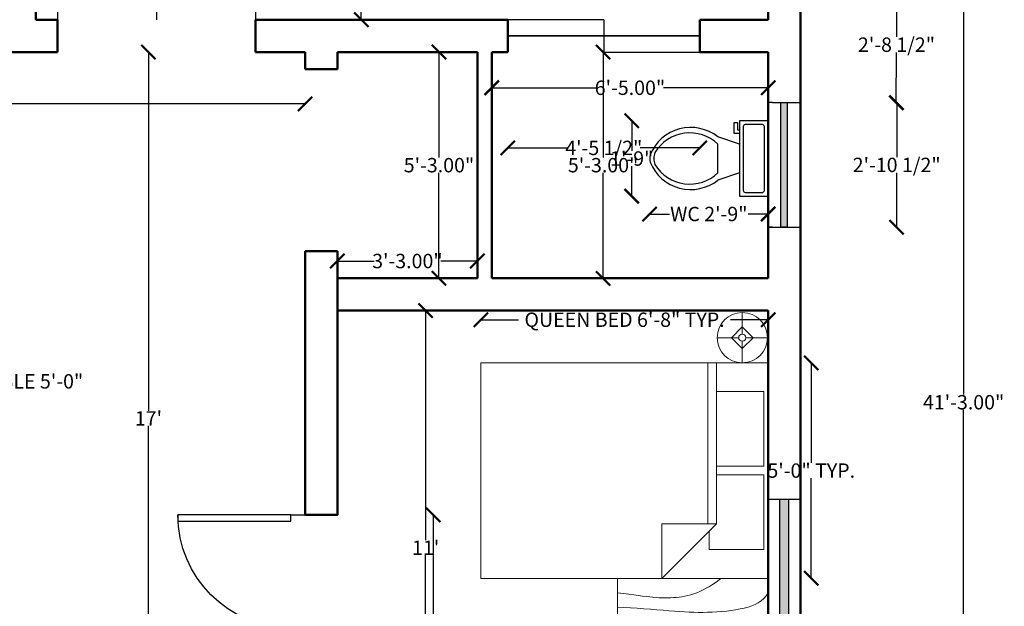
# Model space of a CAD drawing. Units: inches. Extents: x 2466 to 2986, y -30 to 527.
# Tile 4 of 5: x 2711 to 2986, y 190 to 354. Entities that reach past the tile are written whole.
import ezdxf

# ---------------------------------------------------------------- set-up
doc = ezdxf.new("R2010")
doc.units = ezdxf.units.IN
for name, color, linetype, lineweight in [('A-ANNO-DIMS', 2, 'Continuous', 18), ('A-FLOR-FIXT', 8, 'Continuous', 25), ('A-GLAZ', 4, 'Continuous', 25), ('A-GLAZ-PATT', 4, 'Continuous', 13), ('doors', 3, 'Continuous', 25), ('furniture', 6, 'Continuous', 18), ('walls', 40, 'Continuous', 50)]:
    doc.layers.add(name, color=color, linetype=linetype, lineweight=lineweight)
doc.styles.get("Standard").update_dxf_attribs({"font": 'arial.ttf'})
doc.dimstyles.get("Standard").update_dxf_attribs({"dimtxt": 4, "dimasz": 4, "dimexe": 0.18, "dimexo": 0.0625, "dimgap": 0.09, "dimtad": 0, "dimtih": 1, "dimtoh": 1, "dimzin": 0, "dimdsep": 46, "dimlunit": 3, "dimtxsty": 'Standard', "dimblk": 'ARCHTICK', "dimcen": 0.09, "dimse1": 1, "dimse2": 1, "dimclrd": 3, "dimclrt": 2, "dimadec": 0, "dimazin": 0, "dimtfac": 1, "dimtofl": 0, "dimtmove": 0, "dimatfit": 3, "dimfxl": 1, "dimtolj": 1, "dimtzin": 0, "dimarcsym": 0})

# ---------------------------------------------------------------- blocks, each defined once
blk = doc.blocks.new('*U8')
for p, q in [((0, 0), (0, -100)), ((700, 0), (700, -100))]:
    blk.add_line(p, q)
blk.add_lwpolyline([(0, 0), (0, 700), (43.75, 700), (43.75, 0)], close=True)
blk.add_arc((0, 0), 700, 0, 90)
blk = doc.blocks.new('Toilet - top')
for p, q in [((9.5, -6), (9.5, -2)), ((-8, -8.5), (-8, -8)), ((-7, -8), (-7, -9.5)), ((-4, -8), (-6, -14)), ((4, -8), (6, -14)), ((-10, -8.5), (-8, -8.5)), ((-10, -9.5), (-10, -8.5)), ((-7, -9.5), (-10, -9.5)), ((4, -14), (-4, -14))]:
    blk.add_line(p, q)
blk.add_lwpolyline([(10.5, -8), (10.5, 0), (-10.5, 0), (-10.5, -8)], close=True)
for points in [[(-9.5, -2), (-9.5, -6)], [(8.5, -1), (-8.5, -1)], [(-8.5, -7), (8.5, -7)]]:
    blk.add_lwpolyline(points)
for centre, radius, start, end in [((-8.62, -1.88), 0.884, 81.8699, 188.1301), ((8.62, -1.88), 0.884, 351.8699, 98.1301), ((-8.62, -6.12), 0.884, 171.8699, 278.1301), ((8.62, -6.12), 0.884, 261.8699, 8.1301), ((3.52, -21.58), 12.17, 141.4691, 247.9714), ((4.2, -21.82), 11.33, 136.3677, 238.9468), ((-3.52, -21.58), 12.17, 292.0284, 38.5307), ((-4.2, -21.82), 11.33, 301.053, 43.6321), ((0, -27.88), 4, 245.7318, 294.2682), ((0, -29), 4, 254.8605, 285.1395)]:
    blk.add_arc(centre, radius, start, end)
blk = doc.blocks.new('Bed - Queen')
for p, q in [((0, -80.00003), (0, 0)), ((0, 0), (59.99999, 0)), ((59.99999, 0), (59.99999, -80.00003)), ((7.99999, -1.2), (28.79998, -1.2)), ((7.99999, -14.4), (7.99999, -1.2)), ((28.79998, -1.2), (28.79998, -14.4)), ((31.19999, -1.2), (51.99999, -1.2)), ((31.19999, -14.4), (31.19999, -1.2)), ((51.99999, -1.2), (51.99999, -16.4)), ((0, -14.4), (44.8, -14.4)), ((59.99999, -29.6), (44.8, -14.4)), ((44.8, -14.4), (44.8, -29.6)), ((51.99999, -16.4), (46.79936, -16.4)), ((44.8, -16.8), (0, -16.8)), ((44.8, -29.6), (59.99999, -29.6)), ((59.99999, -80.00003), (0, -80.00003))]:
    blk.add_line(p, q)
blk = doc.blocks.new('Lamp - Table')
for p, q in [((0, 7), (0, 1)), ((0, 3), (-3, 0)), ((3, 0), (0, 3)), ((-1, 0), (-7, 0)), ((-3, 0), (0, -3)), ((0, -3), (3, 0)), ((1, 0), (7, 0)), ((0, -1), (0, -7))]:
    blk.add_line(p, q)
for radius in [7, 1]:
    blk.add_circle((0, 0), radius)
blk = doc.blocks.new('Table - Square Woodgrain 42 x 42 in.')
blk.add_line((0, -42), (42, -42))
for points in [[(0, -4), (1.704, -4.2172), (3.2358, -4.4188), (4.615, -4.604), (5.8615, -4.7721), (6.9951, -4.9224), (8.0357, -5.0541), (9.0031, -5.1667), (9.9171, -5.2594), (10.7951, -5.3316), (11.6445, -5.3836), (12.4702, -5.4157), (13.277, -5.4283), (14.0698, -5.4217), (14.8535, -5.3964), (15.6331, -5.3526), (16.4133, -5.2908), (17.1986, -5.2103), (17.9913, -5.1062), (18.793, -4.9727), (19.6056, -4.8038), (20.4307, -4.5937), (21.2701, -4.3365), (22.1256, -4.0262), (22.9989, -3.6571), (23.888, -3.2272), (24.7756, -2.7516), (25.6408, -2.2491), (26.4624, -1.7387), (27.2195, -1.2395), (27.891, -0.7703), (28.456, -0.3501), (28.8934, 0.002)], [(0, -42), (0, 0), (42, 0), (42, -42)], [(0, -8), (1.8203, -8.1001), (3.6741, -8.2149), (5.5411, -8.3408), (7.4011, -8.4741), (9.2339, -8.6112), (11.0193, -8.7484), (12.7371, -8.8821), (14.3671, -9.0086), (15.8954, -9.1246), (17.3337, -9.2278), (18.6997, -9.3159), (20.0116, -9.387), (21.2871, -9.4389), (22.5442, -9.4696), (23.8008, -9.477), (25.0749, -9.459), (26.3791, -9.4137), (27.7049, -9.3403), (29.0383, -9.2382), (30.3655, -9.1068), (31.6728, -8.9455), (32.9461, -8.7535), (34.1717, -8.5304), (35.3358, -8.2756), (36.4268, -7.9863), (37.443, -7.6521), (38.3849, -7.2603), (39.253, -6.7986), (40.048, -6.2542), (40.7705, -5.6147), (41.421, -4.8674), (42, -4)], [(42, -12), (39.1784, -12.8621), (36.4519, -13.5654), (33.8246, -14.1294), (31.3004, -14.5731), (28.8832, -14.9161), (26.577, -15.1775), (24.3858, -15.3768), (22.3136, -15.5332), (20.3622, -15.6632), (18.5254, -15.7718), (16.7947, -15.8612), (15.1618, -15.9338), (13.6183, -15.9916), (12.1558, -16.0369), (10.7659, -16.0718), (9.4403, -16.0987), (8.1703, -16.1191), (6.9461, -16.1325), (5.7577, -16.1377), (4.595, -16.1335), (3.4479, -16.1188), (2.3064, -16.0924), (1.1604, -16.0532), (0, -16)], [(42, -16), (37.6529, -16.7365), (33.8802, -17.329), (30.6179, -17.7961), (27.8015, -18.1561), (25.3668, -18.4275), (23.2497, -18.6288), (21.3859, -18.7785), (19.7111, -18.8949), (18.1693, -18.9939), (16.7375, -19.0795), (15.401, -19.1534), (14.1449, -19.217), (12.9544, -19.2717), (11.8148, -19.3191), (10.7113, -19.3606), (9.6291, -19.3976), (8.5534, -19.4323), (7.47, -19.4689), (6.3643, -19.5122), (5.222, -19.5672), (4.0288, -19.6386), (2.7703, -19.7313), (1.4321, -19.8501), (0, -20)], [(0, -24), (3.9243, -23.6805), (7.4766, -23.4138), (10.6891, -23.1954), (13.5943, -23.0205), (16.2247, -22.8847), (18.6125, -22.7832), (20.7903, -22.7116), (22.7903, -22.6651), (24.6563, -22.642), (26.4764, -22.6507), (28.35, -22.7024), (30.3766, -22.8084), (32.6555, -22.98), (35.2861, -23.2283), (38.3678, -23.5645), (42, -24)], [(42, -32), (37.392, -31.017), (33.4585, -30.2231), (30.1291, -29.5949), (27.3334, -29.109), (25.0009, -28.742), (23.0612, -28.4707), (21.4439, -28.2716), (20.0786, -28.1215), (18.8998, -28.0002), (17.8609, -27.9014), (16.9206, -27.8219), (16.0371, -27.7588), (15.1691, -27.709), (14.2748, -27.6693), (13.3128, -27.6368), (12.2415, -27.6083), (11.0295, -27.5824), (9.6867, -27.5643), (8.233, -27.5608), (6.6884, -27.5787), (5.0728, -27.6248), (3.4062, -27.7058), (1.7086, -27.8286), (0, -28)], [(0, -32), (5.4026, -32.5358), (9.9494, -33.019), (13.7424, -33.4553), (16.8834, -33.8505), (19.4743, -34.2106), (21.6171, -34.5413), (23.4136, -34.8486), (24.9657, -35.1382), (26.3614, -35.4156), (27.6332, -35.6841), (28.7995, -35.9467), (29.8788, -36.2064), (30.8897, -36.4661), (31.8507, -36.7288), (32.7802, -36.9973), (33.6968, -37.2747), (34.6175, -37.5635), (35.5531, -37.8651), (36.5128, -38.1805), (37.506, -38.5108), (38.5421, -38.8568), (39.6302, -39.2197), (40.7797, -39.6004), (42, -40)], [(0, -36), (3.0098, -36.2857), (5.5354, -36.5643), (7.6368, -36.8359), (9.374, -37.1009), (10.807, -37.3597), (11.9957, -37.6126), (13.0002, -37.8599), (13.8804, -38.102), (14.6874, -38.3393), (15.4365, -38.5729), (16.1338, -38.8041), (16.7858, -39.0341), (17.3987, -39.264), (17.9787, -39.4952), (18.5322, -39.7288), (19.0655, -39.9662), (19.5832, -40.2081), (20.0842, -40.4544), (20.5657, -40.7046), (21.0249, -40.9581), (21.459, -41.2144), (21.8653, -41.4731), (22.2409, -41.7335), (22.5831, -41.9951)]]:
    blk.add_lwpolyline(points)
blk = doc.blocks.new('*U18')
for p, q in [((0, 0), (0, -100)), ((800, 0), (800, -100))]:
    blk.add_line(p, q)
blk.add_lwpolyline([(0, 0), (0, 800), (43.75, 800), (43.75, 0)], close=True)
blk.add_arc((0, 0), 800, 0, 90)
blk = doc.blocks.new('_ArchTick')
at = {"color": 0, "linetype": 'ByBlock', "const_width": 0.15}
blk.add_lwpolyline([(-0.5, -0.5), (0.5, 0.5)], dxfattribs=at)
blk = doc.blocks.new('*D22')
at = {"layer": 'A-ANNO-DIMS', "color": 0, "lineweight": -2, "transparency": 16777216}
for p, q in [((2974.18, 494.8), (2974.18, 249.43)), ((2974.18, -0.2), (2974.18, 245.16))]:
    blk.add_line(p, q, dxfattribs=at)
at = {"layer": 'Defpoints', "color": 0, "transparency": 16777216}
for p in [(2928.73, 494.8), (2928.73, -0.2), (2974.18, -0.2)]:
    blk.add_point(p, dxfattribs=at)
at = {"layer": 'A-ANNO-DIMS', "color": 0, "lineweight": -2, "transparency": 16777216, "xscale": 4, "yscale": 4, "zscale": 4}
for p, rotation in [((2974.18, 494.8), 90), ((2974.18, -0.2), 270)]:
    blk.add_blockref('_ArchTick', p, dxfattribs=dict(at, rotation=rotation))
at = {"layer": 'A-ANNO-DIMS', "color": 0, "transparency": 16777216, "insert": (2974.18, 247.3), "char_height": 4, "attachment_point": 5}
blk.add_mtext('\\A1;41\'-3.00"', dxfattribs=at)
blk = doc.blocks.new('*D26')
at = {"layer": 'A-ANNO-DIMS', "color": 0, "lineweight": -2, "transparency": 16777216}
for p, q in [((2806.39, 485.8), (2806.39, 421.89)), ((2806.39, 353.8), (2806.39, 417.7))]:
    blk.add_line(p, q, dxfattribs=at)
at = {"layer": 'Defpoints', "color": 0, "transparency": 16777216}
for p in [(2715.73, 485.8), (2715.73, 353.8), (2806.39, 353.8)]:
    blk.add_point(p, dxfattribs=at)
at = {"layer": 'A-ANNO-DIMS', "color": 0, "lineweight": -2, "transparency": 16777216, "xscale": 4, "yscale": 4, "zscale": 4}
for p, rotation in [((2806.39, 485.8), 90), ((2806.39, 353.8), 270)]:
    blk.add_blockref('_ArchTick', p, dxfattribs=dict(at, rotation=rotation))
at = {"layer": 'A-ANNO-DIMS', "color": 0, "transparency": 16777216, "insert": (2806.39, 419.8), "char_height": 4, "attachment_point": 5}
blk.add_mtext("\\A1;11'", dxfattribs=at)
blk = doc.blocks.new('*D27')
at = {"layer": 'A-ANNO-DIMS', "color": 0, "lineweight": -2, "transparency": 16777216}
for p, q in [((2824.31, 272.8), (2824.31, 208.89)), ((2824.31, 140.8), (2824.31, 204.7))]:
    blk.add_line(p, q, dxfattribs=at)
at = {"layer": 'Defpoints', "color": 0, "transparency": 16777216}
for p in [(2799.73, 272.8), (2824.31, 272.8), (2799.73, 140.8)]:
    blk.add_point(p, dxfattribs=at)
at = {"layer": 'A-ANNO-DIMS', "color": 0, "lineweight": -2, "transparency": 16777216, "xscale": 4, "yscale": 4, "zscale": 4}
for p, rotation in [((2824.31, 272.8), 90), ((2824.31, 140.8), 270)]:
    blk.add_blockref('_ArchTick', p, dxfattribs=dict(at, rotation=rotation))
at = {"layer": 'A-ANNO-DIMS', "color": 0, "transparency": 16777216, "insert": (2824.31, 206.8), "char_height": 4, "attachment_point": 5}
blk.add_mtext("\\A1;11'", dxfattribs=at)
blk = doc.blocks.new('*D29')
at = {"layer": 'A-ANNO-DIMS', "color": 0, "lineweight": -2, "transparency": 16777216}
for p, q in [((2873.75, 344.8), (2873.75, 315.43)), ((2873.75, 281.8), (2873.75, 311.16))]:
    blk.add_line(p, q, dxfattribs=at)
at = {"layer": 'Defpoints', "color": 0, "transparency": 16777216}
for p in [(2842.73, 344.8), (2873.75, 344.8), (2842.73, 281.8)]:
    blk.add_point(p, dxfattribs=at)
at = {"layer": 'A-ANNO-DIMS', "color": 0, "lineweight": -2, "transparency": 16777216, "xscale": 4, "yscale": 4, "zscale": 4}
for p, rotation in [((2873.75, 344.8), 90), ((2873.75, 281.8), 270)]:
    blk.add_blockref('_ArchTick', p, dxfattribs=dict(at, rotation=rotation))
at = {"layer": 'A-ANNO-DIMS', "color": 0, "transparency": 16777216, "insert": (2873.75, 313.3), "char_height": 4, "attachment_point": 5}
blk.add_mtext('\\A1;5\'-3.00"', dxfattribs=at)
blk = doc.blocks.new('*D30')
at = {"layer": 'A-ANNO-DIMS', "color": 0, "lineweight": -2, "transparency": 16777216}
for p, q in [((2842.73, 334.85), (2871.92, 334.85)), ((2919.73, 334.85), (2890.53, 334.85))]:
    blk.add_line(p, q, dxfattribs=at)
at = {"layer": 'Defpoints', "color": 0, "transparency": 16777216}
for p in [(2842.73, 344.8), (2919.73, 344.8), (2842.73, 334.85)]:
    blk.add_point(p, dxfattribs=at)
at = {"layer": 'A-ANNO-DIMS', "color": 0, "lineweight": -2, "transparency": 16777216, "xscale": 4, "yscale": 4, "zscale": 4, "rotation": 180}
blk.add_blockref('_ArchTick', (2842.73, 334.85), dxfattribs=at)
at = {"layer": 'A-ANNO-DIMS', "color": 0, "lineweight": -2, "transparency": 16777216, "xscale": 4, "yscale": 4, "zscale": 4}
blk.add_blockref('_ArchTick', (2919.73, 334.85), dxfattribs=at)
at = {"layer": 'A-ANNO-DIMS', "color": 0, "transparency": 16777216, "insert": (2881.23, 334.85), "char_height": 4, "attachment_point": 5}
blk.add_mtext('\\A1;6\'-5.00"', dxfattribs=at)
blk = doc.blocks.new('*D31')
at = {"layer": 'A-ANNO-DIMS', "color": 0, "lineweight": -2, "transparency": 16777216}
for p, q in [((2828.03, 344.8), (2828.03, 315.43)), ((2828.03, 281.8), (2828.03, 311.16))]:
    blk.add_line(p, q, dxfattribs=at)
at = {"layer": 'Defpoints', "color": 0, "transparency": 16777216}
for p in [(2799.73, 344.8), (2799.73, 281.8), (2828.03, 281.8)]:
    blk.add_point(p, dxfattribs=at)
at = {"layer": 'A-ANNO-DIMS', "color": 0, "lineweight": -2, "transparency": 16777216, "xscale": 4, "yscale": 4, "zscale": 4}
for p, rotation in [((2828.03, 344.8), 90), ((2828.03, 281.8), 270)]:
    blk.add_blockref('_ArchTick', p, dxfattribs=dict(at, rotation=rotation))
at = {"layer": 'A-ANNO-DIMS', "color": 0, "transparency": 16777216, "insert": (2828.03, 313.3), "char_height": 4, "attachment_point": 5}
blk.add_mtext('\\A1;5\'-3.00"', dxfattribs=at)
blk = doc.blocks.new('*D32')
at = {"layer": 'A-ANNO-DIMS', "color": 0, "lineweight": -2, "transparency": 16777216}
for p, q in [((2799.73, 286.61), (2809.94, 286.61)), ((2838.73, 286.61), (2828.51, 286.61))]:
    blk.add_line(p, q, dxfattribs=at)
at = {"layer": 'Defpoints', "color": 0, "transparency": 16777216}
for p in [(2799.73, 286.61), (2799.73, 281.8), (2838.73, 281.8)]:
    blk.add_point(p, dxfattribs=at)
at = {"layer": 'A-ANNO-DIMS', "color": 0, "lineweight": -2, "transparency": 16777216, "xscale": 4, "yscale": 4, "zscale": 4, "rotation": 180}
blk.add_blockref('_ArchTick', (2799.73, 286.61), dxfattribs=at)
at = {"layer": 'A-ANNO-DIMS', "color": 0, "lineweight": -2, "transparency": 16777216, "xscale": 4, "yscale": 4, "zscale": 4}
blk.add_blockref('_ArchTick', (2838.73, 286.61), dxfattribs=at)
at = {"layer": 'A-ANNO-DIMS', "color": 0, "transparency": 16777216, "insert": (2819.23, 286.61), "char_height": 4, "attachment_point": 5}
blk.add_mtext('\\A1;3\'-3.00"', dxfattribs=at)
blk = doc.blocks.new('*D35')
at = {"layer": 'A-ANNO-DIMS', "color": 0, "lineweight": -2, "transparency": 16777216}
for p, q in [((2747.09, 344.8), (2747.09, 244.89)), ((2747.09, 140.8), (2747.09, 240.7))]:
    blk.add_line(p, q, dxfattribs=at)
at = {"layer": 'Defpoints', "color": 0, "transparency": 16777216}
for p in [(2776.87, 344.8), (2747.09, 140.8), (2776.87, 140.8)]:
    blk.add_point(p, dxfattribs=at)
at = {"layer": 'A-ANNO-DIMS', "color": 0, "lineweight": -2, "transparency": 16777216, "xscale": 4, "yscale": 4, "zscale": 4}
for p, rotation in [((2747.09, 344.8), 90), ((2747.09, 140.8), 270)]:
    blk.add_blockref('_ArchTick', p, dxfattribs=dict(at, rotation=rotation))
at = {"layer": 'A-ANNO-DIMS', "color": 0, "transparency": 16777216, "insert": (2747.09, 242.8), "char_height": 4, "attachment_point": 5}
blk.add_mtext("\\A1;17'", dxfattribs=at)
blk = doc.blocks.new('*D36')
at = {"layer": 'A-ANNO-DIMS', "color": 0, "lineweight": -2, "transparency": 16777216}
for p, q in [((2598.73, 330.35), (2691.43, 330.35)), ((2790.73, 330.35), (2698.02, 330.35))]:
    blk.add_line(p, q, dxfattribs=at)
at = {"layer": 'Defpoints', "color": 0, "transparency": 16777216}
for p in [(2598.73, 339.99), (2790.73, 339.99), (2598.73, 330.35)]:
    blk.add_point(p, dxfattribs=at)
at = {"layer": 'A-ANNO-DIMS', "color": 0, "lineweight": -2, "transparency": 16777216, "xscale": 4, "yscale": 4, "zscale": 4, "rotation": 180}
blk.add_blockref('_ArchTick', (2598.73, 330.35), dxfattribs=at)
at = {"layer": 'A-ANNO-DIMS', "color": 0, "lineweight": -2, "transparency": 16777216, "xscale": 4, "yscale": 4, "zscale": 4}
blk.add_blockref('_ArchTick', (2790.73, 330.35), dxfattribs=at)
at = {"layer": 'A-ANNO-DIMS', "color": 0, "transparency": 16777216, "insert": (2694.73, 330.35), "char_height": 4, "attachment_point": 5}
blk.add_mtext("\\A1;16'", dxfattribs=at)
blk = doc.blocks.new('WIN-62_38IN')
h = blk.add_hatch(color=256)
h.dxf.hatch_style = 1
h.paths.add_polyline_path([(3.19, 0), (5.61, 0), (5.61, 62.38), (3.19, 62.38)])
for p, q in [((0, 62.38), (9, 62.38)), ((0, 0), (9, 0))]:
    blk.add_line(p, q)
for points in [[(0, 0), (0, 62.38), (9, 62.38), (9, 62.38), (9, 0)], [(3.19, 0), (3.19, 62.38), (5.61, 62.38), (5.61, 0)]]:
    blk.add_lwpolyline(points, close=True)
blk = doc.blocks.new('*D43')
at = {"layer": 'A-ANNO-DIMS', "color": 3, "lineweight": -2, "transparency": 16777216}
for p, q in [((2839.73, 270.27), (2850.22, 270.27)), ((2919.73, 270.27), (2909.24, 270.27))]:
    blk.add_line(p, q, dxfattribs=at)
at = {"layer": 'Defpoints', "color": 0, "transparency": 16777216}
for p in [(2919.73, 270.27), (2839.73, 258.27), (2919.73, 258.27)]:
    blk.add_point(p, dxfattribs=at)
at = {"layer": 'A-ANNO-DIMS', "color": 3, "lineweight": -2, "transparency": 16777216, "xscale": 4, "yscale": 4, "zscale": 4, "rotation": 180}
blk.add_blockref('_ArchTick', (2839.73, 270.27), dxfattribs=at)
at = {"layer": 'A-ANNO-DIMS', "color": 3, "lineweight": -2, "transparency": 16777216, "xscale": 4, "yscale": 4, "zscale": 4}
blk.add_blockref('_ArchTick', (2919.73, 270.27), dxfattribs=at)
at = {"layer": 'A-ANNO-DIMS', "color": 2, "transparency": 16777216, "insert": (2879.73, 270.27), "char_height": 4, "attachment_point": 5}
blk.add_mtext('\\A1;QUEEN BED 6\'-8" TYP.', dxfattribs=at)
blk = doc.blocks.new('*D44')
at = {"layer": 'A-ANNO-DIMS', "color": 3, "lineweight": -2, "transparency": 16777216}
for p, q in [((2931.73, 258.27), (2931.73, 230.41)), ((2931.73, 198.27), (2931.73, 226.14))]:
    blk.add_line(p, q, dxfattribs=at)
at = {"layer": 'Defpoints', "color": 0, "transparency": 16777216}
for p in [(2919.73, 258.27), (2919.73, 198.27), (2931.73, 198.27)]:
    blk.add_point(p, dxfattribs=at)
at = {"layer": 'A-ANNO-DIMS', "color": 3, "lineweight": -2, "transparency": 16777216, "xscale": 4, "yscale": 4, "zscale": 4}
for p, rotation in [((2931.73, 258.27), 90), ((2931.73, 198.27), 270)]:
    blk.add_blockref('_ArchTick', p, dxfattribs=dict(at, rotation=rotation))
at = {"layer": 'A-ANNO-DIMS', "color": 2, "transparency": 16777216, "insert": (2931.73, 228.27), "char_height": 4, "attachment_point": 5}
blk.add_mtext('\\A1;5\'-0" TYP.', dxfattribs=at)
blk = doc.blocks.new('*D51')
at = {"layer": 'A-ANNO-DIMS', "color": 3, "lineweight": -2, "transparency": 16777216}
for p, q in [((2886.68, 299.7), (2892.28, 299.7)), ((2919.73, 299.7), (2914.12, 299.7))]:
    blk.add_line(p, q, dxfattribs=at)
at = {"layer": 'Defpoints', "color": 0, "transparency": 16777216}
for p in [(2886.68, 304.65), (2919.73, 304.65), (2919.73, 299.7)]:
    blk.add_point(p, dxfattribs=at)
at = {"layer": 'A-ANNO-DIMS', "color": 3, "lineweight": -2, "transparency": 16777216, "xscale": 4, "yscale": 4, "zscale": 4, "rotation": 180}
blk.add_blockref('_ArchTick', (2886.68, 299.7), dxfattribs=at)
at = {"layer": 'A-ANNO-DIMS', "color": 3, "lineweight": -2, "transparency": 16777216, "xscale": 4, "yscale": 4, "zscale": 4}
blk.add_blockref('_ArchTick', (2919.73, 299.7), dxfattribs=at)
at = {"layer": 'A-ANNO-DIMS', "color": 2, "transparency": 16777216, "insert": (2903.2, 299.7), "char_height": 4, "attachment_point": 5}
blk.add_mtext('\\A1;WC 2\'-9"', dxfattribs=at)
blk = doc.blocks.new('*D52')
at = {"layer": 'A-ANNO-DIMS', "color": 3, "lineweight": -2, "transparency": 16777216}
for p, q in [((2881.72, 325.65), (2881.72, 317.29)), ((2881.72, 304.65), (2881.72, 313.02))]:
    blk.add_line(p, q, dxfattribs=at)
at = {"layer": 'Defpoints', "color": 0, "transparency": 16777216}
for p in [(2886.68, 325.65), (2881.72, 304.65), (2886.68, 304.65)]:
    blk.add_point(p, dxfattribs=at)
at = {"layer": 'A-ANNO-DIMS', "color": 3, "lineweight": -2, "transparency": 16777216, "xscale": 4, "yscale": 4, "zscale": 4}
for p, rotation in [((2881.72, 325.65), 90), ((2881.72, 304.65), 270)]:
    blk.add_blockref('_ArchTick', p, dxfattribs=dict(at, rotation=rotation))
at = {"layer": 'A-ANNO-DIMS', "color": 2, "transparency": 16777216, "insert": (2881.72, 315.15), "char_height": 4, "attachment_point": 5}
blk.add_mtext('\\A1;1\'-9"', dxfattribs=at)
blk = doc.blocks.new('*D57')
at = {"layer": 'A-ANNO-DIMS', "color": 3, "lineweight": -2, "transparency": 16777216}
for p, q in [((2703.51, 283.12), (2703.51, 255.28)), ((2703.51, 223.12), (2703.51, 250.96))]:
    blk.add_line(p, q, dxfattribs=at)
at = {"layer": 'Defpoints', "color": 0, "transparency": 16777216}
for p in [(2694.51, 283.12), (2694.51, 223.12), (2703.51, 223.12)]:
    blk.add_point(p, dxfattribs=at)
at = {"layer": 'A-ANNO-DIMS', "color": 3, "lineweight": -2, "transparency": 16777216, "xscale": 4, "yscale": 4, "zscale": 4}
for p, rotation in [((2703.51, 283.12), 90), ((2703.51, 223.12), 270)]:
    blk.add_blockref('_ArchTick', p, dxfattribs=dict(at, rotation=rotation))
at = {"layer": 'A-ANNO-DIMS', "color": 2, "transparency": 16777216, "insert": (2703.51, 253.12), "char_height": 4, "attachment_point": 5}
blk.add_mtext('\\A1;COFFEE TABLE 5\'-0"', dxfattribs=at)
blk = doc.blocks.new('*D64')
at = {"layer": 'A-ANNO-DIMS', "color": 3, "lineweight": -2, "transparency": 16777216}
for p, q in [((2826.43, 215.94), (2826.43, 186.57)), ((2826.43, 152.94), (2826.43, 182.31))]:
    blk.add_line(p, q, dxfattribs=at)
at = {"layer": 'Defpoints', "color": 0, "transparency": 16777216}
for p in [(2799.73, 215.94), (2799.73, 152.94), (2826.43, 152.94)]:
    blk.add_point(p, dxfattribs=at)
at = {"layer": 'A-ANNO-DIMS', "color": 3, "lineweight": -2, "transparency": 16777216, "xscale": 4, "yscale": 4, "zscale": 4}
for p, rotation in [((2826.43, 215.94), 90), ((2826.43, 152.94), 270)]:
    blk.add_blockref('_ArchTick', p, dxfattribs=dict(at, rotation=rotation))
at = {"layer": 'A-ANNO-DIMS', "color": 2, "transparency": 16777216, "insert": (2826.43, 184.44), "char_height": 4, "attachment_point": 5}
blk.add_mtext('\\A1;5\'-3"', dxfattribs=at)
blk = doc.blocks.new('*D65')
at = {"layer": 'A-ANNO-DIMS', "color": 3, "lineweight": -2, "transparency": 16777216}
for p, q in [((2847.17, 318.1), (2863.79, 318.1)), ((2900.7, 318.1), (2884.08, 318.1))]:
    blk.add_line(p, q, dxfattribs=at)
at = {"layer": 'Defpoints', "color": 0, "transparency": 16777216}
for p in [(2847.17, 344.8), (2900.7, 344.8), (2847.17, 318.1)]:
    blk.add_point(p, dxfattribs=at)
at = {"layer": 'A-ANNO-DIMS', "color": 3, "lineweight": -2, "transparency": 16777216, "xscale": 4, "yscale": 4, "zscale": 4, "rotation": 180}
blk.add_blockref('_ArchTick', (2847.17, 318.1), dxfattribs=at)
at = {"layer": 'A-ANNO-DIMS', "color": 3, "lineweight": -2, "transparency": 16777216, "xscale": 4, "yscale": 4, "zscale": 4}
blk.add_blockref('_ArchTick', (2900.7, 318.1), dxfattribs=at)
at = {"layer": 'A-ANNO-DIMS', "color": 2, "transparency": 16777216, "insert": (2873.94, 318.1), "char_height": 4, "attachment_point": 5}
blk.add_mtext('\\A1;4\'-5 1/2"', dxfattribs=at)
blk = doc.blocks.new('*D67')
at = {"layer": 'A-ANNO-DIMS', "color": 3, "lineweight": -2, "transparency": 16777216}
for p, q in [((2888.73, 521.5), (2901.32, 521.5)), ((2924.73, 521.5), (2912.13, 521.5))]:
    blk.add_line(p, q, dxfattribs=at)
at = {"layer": 'Defpoints', "color": 0, "transparency": 16777216}
for p in [(2924.73, 521.5), (2888.73, 47.8), (2924.73, 47.8)]:
    blk.add_point(p, dxfattribs=at)
at = {"layer": 'A-ANNO-DIMS', "color": 3, "lineweight": -2, "transparency": 16777216, "xscale": 4, "yscale": 4, "zscale": 4, "rotation": 180}
blk.add_blockref('_ArchTick', (2888.73, 521.5), dxfattribs=at)
at = {"layer": 'A-ANNO-DIMS', "color": 3, "lineweight": -2, "transparency": 16777216, "xscale": 4, "yscale": 4, "zscale": 4}
blk.add_blockref('_ArchTick', (2924.73, 521.5), dxfattribs=at)
at = {"layer": 'A-ANNO-DIMS', "color": 2, "transparency": 16777216, "insert": (2906.73, 521.5), "char_height": 4, "attachment_point": 5}
blk.add_mtext('\\A1;3\'-0"', dxfattribs=at)
blk = doc.blocks.new('*D70')
at = {"layer": 'A-ANNO-DIMS', "color": 3, "lineweight": -2, "transparency": 16777216}
for p, q in [((2859.73, 521.5), (2882.24, 521.5)), ((2915.73, 521.5), (2893.21, 521.5))]:
    blk.add_line(p, q, dxfattribs=at)
at = {"layer": 'Defpoints', "color": 0, "transparency": 16777216}
for p in [(2915.73, 521.5), (2859.73, 140.8), (2915.73, 140.8)]:
    blk.add_point(p, dxfattribs=at)
at = {"layer": 'A-ANNO-DIMS', "color": 3, "lineweight": -2, "transparency": 16777216, "xscale": 4, "yscale": 4, "zscale": 4, "rotation": 180}
blk.add_blockref('_ArchTick', (2859.73, 521.5), dxfattribs=at)
at = {"layer": 'A-ANNO-DIMS', "color": 3, "lineweight": -2, "transparency": 16777216, "xscale": 4, "yscale": 4, "zscale": 4}
blk.add_blockref('_ArchTick', (2915.73, 521.5), dxfattribs=at)
at = {"layer": 'A-ANNO-DIMS', "color": 2, "transparency": 16777216, "insert": (2887.73, 521.5), "char_height": 4, "attachment_point": 5}
blk.add_mtext('\\A1;4\'-8"', dxfattribs=at)
blk = doc.blocks.new('*D71')
at = {"layer": 'A-ANNO-DIMS', "color": 3, "lineweight": -2, "transparency": 16777216}
for p, q in [((2955.53, 330.72), (2955.53, 315.53)), ((2955.53, 296.02), (2955.53, 311.21))]:
    blk.add_line(p, q, dxfattribs=at)
at = {"layer": 'Defpoints', "color": 0, "transparency": 16777216}
for p in [(2928.73, 330.72), (2955.53, 330.72), (2928.73, 296.02)]:
    blk.add_point(p, dxfattribs=at)
at = {"layer": 'A-ANNO-DIMS', "color": 3, "lineweight": -2, "transparency": 16777216, "xscale": 4, "yscale": 4, "zscale": 4}
for p, rotation in [((2955.53, 330.72), 90), ((2955.53, 296.02), 270)]:
    blk.add_blockref('_ArchTick', p, dxfattribs=dict(at, rotation=rotation))
at = {"layer": 'A-ANNO-DIMS', "color": 2, "transparency": 16777216, "insert": (2955.53, 313.37), "char_height": 4, "attachment_point": 5}
blk.add_mtext('\\A1;2\'-10 1/2"', dxfattribs=at)
blk = doc.blocks.new('*D83')
at = {"layer": 'A-ANNO-DIMS', "color": 3, "lineweight": -2, "transparency": 16777216}
for p, q in [((2955.53, 363.07), (2955.48, 349.01)), ((2955.43, 330.64), (2955.47, 344.7))]:
    blk.add_line(p, q, dxfattribs=at)
at = {"layer": 'Defpoints', "color": 0, "transparency": 16777216}
for p in [(2928.83, 363.15), (2928.73, 330.72), (2955.43, 330.64)]:
    blk.add_point(p, dxfattribs=at)
at = {"layer": 'A-ANNO-DIMS', "color": 3, "lineweight": -2, "transparency": 16777216, "xscale": 4, "yscale": 4, "zscale": 4}
for p, rotation in [((2955.53, 363.07), 89.81962137861794), ((2955.43, 330.64), 269.8196213786179)]:
    blk.add_blockref('_ArchTick', p, dxfattribs=dict(at, rotation=rotation))
at = {"layer": 'A-ANNO-DIMS', "color": 2, "transparency": 16777216, "insert": (2955.48, 346.85), "char_height": 4, "attachment_point": 5}
blk.add_mtext('\\A1;2\'-8 1/2"', dxfattribs=at)

msp = doc.modelspace()

# ---------------------------------------------------------------- hatches: boundary and pattern name
at = {"layer": 'A-GLAZ-PATT'}
h = msp.add_hatch(color=256, dxfattribs=at)
h.dxf.hatch_style = 1
h.paths.add_polyline_path([(2923.251, 296.019), (2924.996, 296.019), (2924.996, 330.723), (2923.251, 330.723)])

# ---------------------------------------------------------------- linework, layer by layer
at = {"layer": 'A-GLAZ'}
for p, q in [((2920.944, 330.723), (2919.725, 330.723)), ((2920.944, 330.723), (2927.451, 330.723)), ((2927.451, 330.723), (2928.725, 330.723)), ((2920.944, 296.019), (2919.725, 296.019)), ((2919.725, 296.019), (2928.725, 296.019)), ((2920.944, 296.019), (2927.451, 296.019))]:
    msp.add_line(p, q, dxfattribs=at)
msp.add_lwpolyline([(2923.251, 296.019), (2923.251, 330.723), (2924.996, 330.723), (2924.996, 296.019)], close=True, dxfattribs=at)
at = {"layer": 'doors'}
msp.add_line((2873.937, 353.795), (2873.937, 344.795), dxfattribs=at)
for points in [[(2873.937, 353.795), (2847.174, 353.795), (2847.174, 349.295), (2900.701, 349.295), (2900.701, 353.795)], [(2873.937, 344.795), (2900.701, 344.795), (2900.701, 349.295), (2847.174, 349.295), (2847.174, 344.795)]]:
    msp.add_lwpolyline(points, dxfattribs=at)
at = {"layer": 'walls'}
for p, q in [((2928.725, 494.795), (2928.725, 131.795)), ((2715.725, 485.795), (2715.725, 353.795)), ((2919.725, 485.795), (2919.725, 353.795)), ((2715.725, 353.795), (2721.753, 353.795)), ((2721.753, 353.795), (2721.753, 344.795)), ((2776.871, 353.795), (2847.174, 353.795)), ((2776.871, 353.795), (2776.871, 344.795)), ((2847.174, 353.795), (2847.174, 344.795)), ((2900.701, 353.795), (2900.701, 344.795)), ((2900.701, 353.795), (2919.725, 353.795)), ((2688.139, 344.795), (2721.753, 344.795)), ((2776.871, 344.795), (2790.725, 344.795)), ((2790.725, 344.795), (2790.725, 339.988)), ((2799.725, 344.795), (2799.725, 339.988)), ((2799.725, 344.795), (2838.725, 344.795)), ((2838.725, 344.795), (2838.725, 281.795)), ((2842.725, 344.795), (2842.725, 281.795)), ((2842.725, 344.795), (2847.174, 344.795)), ((2900.701, 344.795), (2919.725, 344.795)), ((2919.725, 344.795), (2919.725, 281.795)), ((2799.725, 339.988), (2790.725, 339.988)), ((2799.725, 289.328), (2790.725, 289.328)), ((2799.725, 281.795), (2838.725, 281.795)), ((2842.725, 281.795), (2919.725, 281.795)), ((2799.725, 272.795), (2838.725, 272.795)), ((2799.725, 272.795), (2919.725, 272.795)), ((2842.725, 272.795), (2919.725, 272.795)), ((2919.725, 272.795), (2919.725, 140.795))]:
    msp.add_line(p, q, dxfattribs=at)
msp.add_lwpolyline([(2790.725, 289.328), (2790.725, 215.936), (2799.725, 215.936), (2799.725, 289.328)], dxfattribs=at)

# ---------------------------------------------------------------- block references
at = {"layer": 'A-FLOR-FIXT', "rotation": 270}
msp.add_blockref('Toilet - top', (2919.725, 315.154), dxfattribs=at)
at = {"layer": 'A-GLAZ'}
msp.add_blockref('WIN-62_38IN', (2919.828, 157.909), dxfattribs=at)
at = {"layer": 'doors', "yscale": 0.0393700787401575, "zscale": 0.0393700787401575}
for p, xscale in [((2721.753, 357.732), 0.0393700787401575), ((2776.871, 357.732), -0.0393700787401575)]:
    msp.add_blockref('*U8', p, dxfattribs=dict(at, xscale=xscale))
at = {"layer": 'doors', "xscale": -0.0393700787401575, "yscale": 0.0393700787401575, "zscale": 0.0393700787401575, "rotation": 90}
msp.add_blockref('*U18', (2786.788, 215.936), dxfattribs=at)
at = {"layer": 'furniture'}
for name, p in [('Lamp - Table', (2912.525, 265.274)), ('Table - Square Woodgrain 42 x 42 in.', (2877.725, 198.274))]:
    msp.add_blockref(name, p, dxfattribs=at)
at = {"layer": 'furniture', "rotation": 270}
msp.add_blockref('Bed - Queen', (2919.725, 258.274), dxfattribs=at)

# ---------------------------------------------------------------- dimensions: what is measured, and where the dimension line sits
at = {"layer": 'A-ANNO-DIMS'}
for base, p1, p2, override, picture, middle in [((2915.725, 521.495), (2859.725, 140.795), (2915.725, 140.795), {"dimdec": 1, "dimlfac": 1, "dimrnd": 0, "dimzin": 1, "dimdsep": 46, "dimlunit": 4, "dimfrac": 2}, '*D70', (2887.725, 521.495)), ((2924.725, 521.495), (2888.725, 47.795), (2924.725, 47.795), {"dimdec": 1, "dimlfac": 1, "dimrnd": 0, "dimzin": 1, "dimdsep": 46, "dimlunit": 4, "dimfrac": 2}, '*D67', (2906.725, 521.495)), ((2842.725, 334.848), (2919.725, 344.795), (2842.725, 344.795), {"dimclrd": 0, "dimclre": 0, "dimclrt": 0}, '*D30', (2881.225, 334.848)), ((2598.725, 330.35), (2790.725, 339.988), (2598.725, 339.988), {"dimclrd": 0, "dimclre": 0, "dimclrt": 0}, '*D36', (2694.725, 330.35)), ((2799.725, 286.605), (2838.725, 281.795), (2799.725, 281.795), {"dimclrd": 0, "dimclre": 0, "dimclrt": 0}, '*D32', (2819.225, 286.605))]:
    dim = msp.add_linear_dim(base=base, p1=p1, p2=p2, dimstyle='Standard', override=override, dxfattribs=at)
    dim.commit()
    dim.dimension.update_dxf_attribs({"geometry": picture, "text_midpoint": middle})
for base, p1, p2, angle, override, picture, middle in [((2974.184, -0.205), (2928.725, 494.795), (2928.725, -0.205), 90, {"dimclrd": 0, "dimclre": 0, "dimclrt": 0}, '*D22', (2974.184, 247.295)), ((2806.394, 353.795), (2715.725, 485.795), (2715.725, 353.795), 90, {"dimclrd": 0, "dimclre": 0, "dimclrt": 0}, '*D26', (2806.394, 419.795)), ((2955.425, 330.639), (2928.828, 363.154), (2928.725, 330.723), 269.81962, {"dimdec": 1, "dimlfac": 1, "dimrnd": 0, "dimzin": 1, "dimdsep": 46, "dimlunit": 4, "dimfrac": 2}, '*D83', (2955.476, 346.854)), ((2747.088, 140.795), (2776.871, 344.795), (2776.871, 140.795), 90, {"dimclrd": 0, "dimclre": 0, "dimclrt": 0}, '*D35', (2747.088, 242.795)), ((2828.027, 281.795), (2799.725, 344.795), (2799.725, 281.795), 90, {"dimclrd": 0, "dimclre": 0, "dimclrt": 0}, '*D31', (2828.027, 313.295)), ((2873.747, 344.795), (2842.725, 281.795), (2842.725, 344.795), 90, {"dimclrd": 0, "dimclre": 0, "dimclrt": 0}, '*D29', (2873.747, 313.295)), ((2847.174, 318.095), (2900.701, 344.795), (2847.174, 344.795), 180, {"dimdec": 1, "dimlfac": 1, "dimrnd": 0, "dimzin": 1, "dimdsep": 46, "dimlunit": 4, "dimfrac": 2}, '*D65', (2873.937, 318.095)), ((2955.528, 330.723), (2928.725, 296.019), (2928.725, 330.723), 90, {"dimdec": 1, "dimlfac": 1, "dimrnd": 0, "dimzin": 1, "dimdsep": 46, "dimlunit": 4, "dimfrac": 2}, '*D71', (2955.528, 313.371)), ((2881.722, 304.654), (2886.679, 325.654), (2886.679, 304.654), 270, {"dimdec": 1, "dimlfac": 1, "dimrnd": 0, "dimzin": 1, "dimdsep": 46, "dimlunit": 4, "dimfrac": 2}, '*D52', (2881.722, 315.154)), ((2824.314, 272.795), (2799.725, 140.795), (2799.725, 272.795), 90, {"dimclrd": 0, "dimclre": 0, "dimclrt": 0}, '*D27', (2824.314, 206.795)), ((2826.425, 152.944), (2799.725, 215.936), (2799.725, 152.944), 270, {"dimdec": 1, "dimlfac": 1, "dimrnd": 0, "dimzin": 1, "dimdsep": 46, "dimlunit": 4, "dimfrac": 2}, '*D64', (2826.425, 184.44))]:
    dim = msp.add_linear_dim(base=base, p1=p1, p2=p2, angle=angle, dimstyle='Standard', override=override, dxfattribs=at)
    dim.commit()
    dim.dimension.update_dxf_attribs({"geometry": picture, "text_midpoint": middle})
for base, p1, p2, text, picture, middle in [((2919.725, 299.697), (2886.679, 304.654), (2919.725, 304.654), 'WC <>', '*D51', (2903.202, 299.697)), ((2919.725, 270.274), (2839.725, 258.274), (2919.725, 258.274), 'QUEEN BED <> TYP.', '*D43', (2879.725, 270.274))]:
    dim = msp.add_linear_dim(base=base, p1=p1, p2=p2, text=text, dimstyle='Standard', override={"dimdec": 1, "dimlfac": 1, "dimrnd": 0, "dimzin": 1, "dimdsep": 46, "dimlunit": 4, "dimfrac": 2}, dxfattribs=at)
    dim.commit()
    dim.dimension.update_dxf_attribs({"geometry": picture, "text_midpoint": middle})
for base, p1, p2, text, picture, middle in [((2703.512, 223.123), (2694.512, 283.123), (2694.512, 223.123), 'COFFEE TABLE <>', '*D57', (2703.512, 253.123)), ((2931.725, 198.274), (2919.725, 258.274), (2919.725, 198.274), '<> TYP.', '*D44', (2931.725, 228.274))]:
    dim = msp.add_linear_dim(base=base, p1=p1, p2=p2, angle=270, text=text, dimstyle='Standard', override={"dimdec": 1, "dimlfac": 1, "dimrnd": 0, "dimzin": 1, "dimdsep": 46, "dimlunit": 4, "dimfrac": 2}, dxfattribs=at)
    dim.commit()
    dim.dimension.update_dxf_attribs({"geometry": picture, "text_midpoint": middle})

doc.saveas('drawing.dxf')
